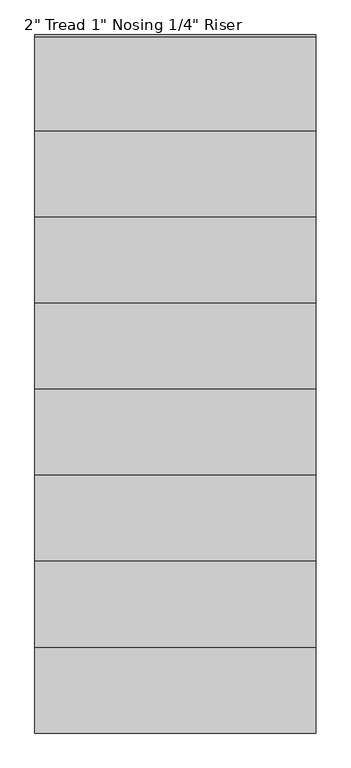
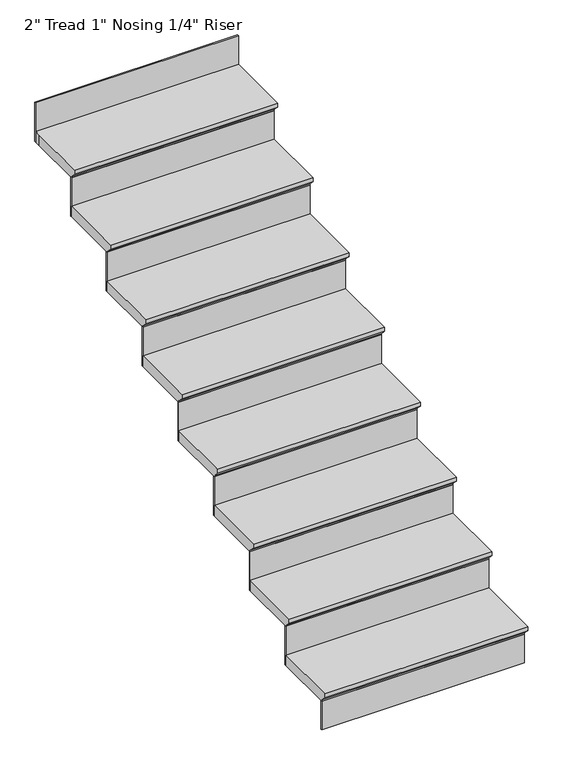
"""IFC4 building model written with IfcOpenShell, lengths in millimetres: stair flight geometry."""

from ifc_helpers import new_model, si_unit, origin, place, context, project, spatial, faceted_brep, source, transform, mapped, element, save


def stair_flight_c2955f1a(model_context):
    return source(origin(), model_context, "Body", "Brep", [
        faceted_brep([(-6758.2994093, 3499.0237487, 167.9863636), (-6758.2994093, 3499.0237487, 187.0363636), (-7672.6994093, 3499.0237487, 187.0363636), (-7672.6994093, 3499.0237487, 167.9863636), (-6758.2994093, 3524.4237487, 142.5863636), (-7672.6994093, 3524.4237487, 142.5863636), (-6758.2994093, 3803.8237487, 187.0363636), (-7672.6994093, 3803.8237487, 187.0363636), (-7672.6994093, 3524.4237487, 136.2363636), (-7672.6994093, 3803.8237487, 136.2363636), (-6758.2994093, 3803.8237487, 136.2363636), (-6758.2994093, 3524.4237487, 136.2363636)], [[[0, 1, 2, 3]], [[4, 0, 3, 5]], [[2, 1, 6, 7]], [[8, 9, 10, 11]], [[2, 7, 9, 8, 5, 3]], [[8, 11, 4, 5]], [[6, 1, 0, 4, 11, 10]], [[7, 6, 10, 9]]]),
        faceted_brep([(-6758.2994093, 3524.4237487, 136.2363636), (-6758.2994093, 3524.4237487, 0.0), (-6758.2994093, 3530.7737487, 0.0), (-6758.2994093, 3530.7737487, 136.2363636), (-7672.6994093, 3524.4237487, 136.2363636), (-7672.6994093, 3530.7737487, 136.2363636), (-7672.6994093, 3530.7737487, 0.0), (-7672.6994093, 3524.4237487, 0.0)], [[[0, 1, 2, 3]], [[4, 5, 6, 7]], [[1, 0, 4, 7]], [[2, 1, 7, 6]], [[3, 2, 6, 5]], [[0, 3, 5, 4]]]),
        faceted_brep([(-6758.2994093, 3803.8237487, 323.2727273), (-6758.2994093, 3803.8237487, 136.2363636), (-6758.2994093, 3810.1737487, 136.2363636), (-6758.2994093, 3810.1737487, 323.2727273), (-7672.6994093, 3803.8237487, 323.2727273), (-7672.6994093, 3810.1737487, 323.2727273), (-7672.6994093, 3810.1737487, 136.2363636), (-7672.6994093, 3803.8237487, 136.2363636)], [[[0, 1, 2, 3]], [[4, 5, 6, 7]], [[1, 0, 4, 7]], [[2, 1, 7, 6]], [[3, 2, 6, 5]], [[0, 3, 5, 4]]]),
        faceted_brep([(-7672.6994093, 3778.4237487, 374.0727273), (-6758.2994093, 3778.4237487, 374.0727273), (-6758.2994093, 4083.2237487, 374.0727273), (-7672.6994093, 4083.2237487, 374.0727273), (-7672.6994093, 3803.8237487, 323.2727273), (-7672.6994093, 4083.2237487, 323.2727273), (-6758.2994093, 4083.2237487, 323.2727273), (-6758.2994093, 3803.8237487, 323.2727273), (-7672.6994093, 3803.8237487, 329.6227273), (-7672.6994093, 3778.4237487, 355.0227273), (-6758.2994093, 3803.8237487, 329.6227273), (-6758.2994093, 3778.4237487, 355.0227273)], [[[0, 1, 2, 3]], [[4, 5, 6, 7]], [[0, 3, 5, 4, 8, 9]], [[4, 7, 10, 8]], [[2, 1, 11, 10, 7, 6]], [[3, 2, 6, 5]], [[11, 1, 0, 9]], [[10, 11, 9, 8]]]),
        faceted_brep([(-6758.2994093, 4083.2237487, 510.3090909), (-6758.2994093, 4083.2237487, 323.2727273), (-6758.2994093, 4089.5737487, 323.2727273), (-6758.2994093, 4089.5737487, 510.3090909), (-7672.6994093, 4083.2237487, 510.3090909), (-7672.6994093, 4089.5737487, 510.3090909), (-7672.6994093, 4089.5737487, 323.2727273), (-7672.6994093, 4083.2237487, 323.2727273)], [[[0, 1, 2, 3]], [[4, 5, 6, 7]], [[1, 0, 4, 7]], [[2, 1, 7, 6]], [[3, 2, 6, 5]], [[0, 3, 5, 4]]]),
        faceted_brep([(-7672.6994093, 4057.8237487, 561.1090909), (-6758.2994093, 4057.8237487, 561.1090909), (-6758.2994093, 4362.6237487, 561.1090909), (-7672.6994093, 4362.6237487, 561.1090909), (-7672.6994093, 4083.2237487, 510.3090909), (-7672.6994093, 4362.6237487, 510.3090909), (-6758.2994093, 4362.6237487, 510.3090909), (-6758.2994093, 4083.2237487, 510.3090909), (-7672.6994093, 4083.2237487, 516.6590909), (-7672.6994093, 4057.8237487, 542.0590909), (-6758.2994093, 4083.2237487, 516.6590909), (-6758.2994093, 4057.8237487, 542.0590909)], [[[0, 1, 2, 3]], [[4, 5, 6, 7]], [[0, 3, 5, 4, 8, 9]], [[4, 7, 10, 8]], [[2, 1, 11, 10, 7, 6]], [[3, 2, 6, 5]], [[11, 1, 0, 9]], [[10, 11, 9, 8]]]),
        faceted_brep([(-6758.2994093, 4362.6237487, 697.3454545), (-6758.2994093, 4362.6237487, 510.3090909), (-6758.2994093, 4368.9737487, 510.3090909), (-6758.2994093, 4368.9737487, 697.3454545), (-7672.6994093, 4362.6237487, 697.3454545), (-7672.6994093, 4368.9737487, 697.3454545), (-7672.6994093, 4368.9737487, 510.3090909), (-7672.6994093, 4362.6237487, 510.3090909)], [[[0, 1, 2, 3]], [[4, 5, 6, 7]], [[1, 0, 4, 7]], [[2, 1, 7, 6]], [[3, 2, 6, 5]], [[0, 3, 5, 4]]]),
        faceted_brep([(-7672.6994093, 4337.2237487, 748.1454545), (-6758.2994093, 4337.2237487, 748.1454545), (-6758.2994093, 4642.0237487, 748.1454545), (-7672.6994093, 4642.0237487, 748.1454545), (-7672.6994093, 4362.6237487, 697.3454545), (-7672.6994093, 4642.0237487, 697.3454545), (-6758.2994093, 4642.0237487, 697.3454545), (-6758.2994093, 4362.6237487, 697.3454545), (-7672.6994093, 4362.6237487, 703.6954545), (-7672.6994093, 4337.2237487, 729.0954545), (-6758.2994093, 4362.6237487, 703.6954545), (-6758.2994093, 4337.2237487, 729.0954545)], [[[0, 1, 2, 3]], [[4, 5, 6, 7]], [[0, 3, 5, 4, 8, 9]], [[4, 7, 10, 8]], [[2, 1, 11, 10, 7, 6]], [[3, 2, 6, 5]], [[11, 1, 0, 9]], [[10, 11, 9, 8]]]),
        faceted_brep([(-6758.2994093, 4642.0237487, 884.3818182), (-6758.2994093, 4642.0237487, 697.3454545), (-6758.2994093, 4648.3737487, 697.3454545), (-6758.2994093, 4648.3737487, 884.3818182), (-7672.6994093, 4642.0237487, 884.3818182), (-7672.6994093, 4648.3737487, 884.3818182), (-7672.6994093, 4648.3737487, 697.3454545), (-7672.6994093, 4642.0237487, 697.3454545)], [[[0, 1, 2, 3]], [[4, 5, 6, 7]], [[1, 0, 4, 7]], [[2, 1, 7, 6]], [[3, 2, 6, 5]], [[0, 3, 5, 4]]]),
        faceted_brep([(-7672.6994093, 4616.6237487, 935.1818182), (-6758.2994093, 4616.6237487, 935.1818182), (-6758.2994093, 4921.4237487, 935.1818182), (-7672.6994093, 4921.4237487, 935.1818182), (-7672.6994093, 4642.0237487, 884.3818182), (-7672.6994093, 4921.4237487, 884.3818182), (-6758.2994093, 4921.4237487, 884.3818182), (-6758.2994093, 4642.0237487, 884.3818182), (-7672.6994093, 4642.0237487, 890.7318182), (-7672.6994093, 4616.6237487, 916.1318182), (-6758.2994093, 4642.0237487, 890.7318182), (-6758.2994093, 4616.6237487, 916.1318182)], [[[0, 1, 2, 3]], [[4, 5, 6, 7]], [[0, 3, 5, 4, 8, 9]], [[4, 7, 10, 8]], [[2, 1, 11, 10, 7, 6]], [[3, 2, 6, 5]], [[11, 1, 0, 9]], [[10, 11, 9, 8]]]),
        faceted_brep([(-6758.2994093, 4921.4237487, 1071.4181818), (-6758.2994093, 4921.4237487, 884.3818182), (-6758.2994093, 4927.7737487, 884.3818182), (-6758.2994093, 4927.7737487, 1071.4181818), (-7672.6994093, 4921.4237487, 1071.4181818), (-7672.6994093, 4927.7737487, 1071.4181818), (-7672.6994093, 4927.7737487, 884.3818182), (-7672.6994093, 4921.4237487, 884.3818182)], [[[0, 1, 2, 3]], [[4, 5, 6, 7]], [[1, 0, 4, 7]], [[2, 1, 7, 6]], [[3, 2, 6, 5]], [[0, 3, 5, 4]]]),
        faceted_brep([(-7672.6994093, 4896.0237487, 1122.2181818), (-6758.2994093, 4896.0237487, 1122.2181818), (-6758.2994093, 5200.8237487, 1122.2181818), (-7672.6994093, 5200.8237487, 1122.2181818), (-7672.6994093, 4921.4237487, 1071.4181818), (-7672.6994093, 5200.8237487, 1071.4181818), (-6758.2994093, 5200.8237487, 1071.4181818), (-6758.2994093, 4921.4237487, 1071.4181818), (-7672.6994093, 4921.4237487, 1077.7681818), (-7672.6994093, 4896.0237487, 1103.1681818), (-6758.2994093, 4921.4237487, 1077.7681818), (-6758.2994093, 4896.0237487, 1103.1681818)], [[[0, 1, 2, 3]], [[4, 5, 6, 7]], [[0, 3, 5, 4, 8, 9]], [[4, 7, 10, 8]], [[2, 1, 11, 10, 7, 6]], [[3, 2, 6, 5]], [[11, 1, 0, 9]], [[10, 11, 9, 8]]]),
        faceted_brep([(-6758.2994093, 5200.8237487, 1258.4545455), (-6758.2994093, 5200.8237487, 1071.4181818), (-6758.2994093, 5207.1737487, 1071.4181818), (-6758.2994093, 5207.1737487, 1258.4545455), (-7672.6994093, 5200.8237487, 1258.4545455), (-7672.6994093, 5207.1737487, 1258.4545455), (-7672.6994093, 5207.1737487, 1071.4181818), (-7672.6994093, 5200.8237487, 1071.4181818)], [[[0, 1, 2, 3]], [[4, 5, 6, 7]], [[1, 0, 4, 7]], [[2, 1, 7, 6]], [[3, 2, 6, 5]], [[0, 3, 5, 4]]]),
        faceted_brep([(-7672.6994093, 5175.4237487, 1309.2545455), (-6758.2994093, 5175.4237487, 1309.2545455), (-6758.2994093, 5480.2237487, 1309.2545455), (-7672.6994093, 5480.2237487, 1309.2545455), (-7672.6994093, 5200.8237487, 1258.4545455), (-7672.6994093, 5480.2237487, 1258.4545455), (-6758.2994093, 5480.2237487, 1258.4545455), (-6758.2994093, 5200.8237487, 1258.4545455), (-7672.6994093, 5200.8237487, 1264.8045455), (-7672.6994093, 5175.4237487, 1290.2045455), (-6758.2994093, 5200.8237487, 1264.8045455), (-6758.2994093, 5175.4237487, 1290.2045455)], [[[0, 1, 2, 3]], [[4, 5, 6, 7]], [[0, 3, 5, 4, 8, 9]], [[4, 7, 10, 8]], [[2, 1, 11, 10, 7, 6]], [[3, 2, 6, 5]], [[11, 1, 0, 9]], [[10, 11, 9, 8]]]),
        faceted_brep([(-6758.2994093, 5759.6237487, 1632.5272727), (-6758.2994093, 5759.6237487, 1445.4909091), (-6758.2994093, 5765.9737487, 1445.4909091), (-6758.2994093, 5765.9737487, 1632.5272727), (-7672.6994093, 5759.6237487, 1632.5272727), (-7672.6994093, 5765.9737487, 1632.5272727), (-7672.6994093, 5765.9737487, 1445.4909091), (-7672.6994093, 5759.6237487, 1445.4909091)], [[[0, 1, 2, 3]], [[4, 5, 6, 7]], [[1, 0, 4, 7]], [[2, 1, 7, 6]], [[3, 2, 6, 5]], [[0, 3, 5, 4]]]),
        faceted_brep([(-6758.2994093, 5480.2237487, 1445.4909091), (-6758.2994093, 5480.2237487, 1258.4545455), (-6758.2994093, 5486.5737487, 1258.4545455), (-6758.2994093, 5486.5737487, 1445.4909091), (-7672.6994093, 5480.2237487, 1445.4909091), (-7672.6994093, 5486.5737487, 1445.4909091), (-7672.6994093, 5486.5737487, 1258.4545455), (-7672.6994093, 5480.2237487, 1258.4545455)], [[[0, 1, 2, 3]], [[4, 5, 6, 7]], [[1, 0, 4, 7]], [[2, 1, 7, 6]], [[3, 2, 6, 5]], [[0, 3, 5, 4]]]),
        faceted_brep([(-7672.6994093, 5759.6237487, 1496.2909091), (-7672.6994093, 5734.2237487, 1496.2909091), (-7672.6994093, 5454.8237487, 1496.2909091), (-6758.2994093, 5454.8237487, 1496.2909091), (-6758.2994093, 5759.6237487, 1496.2909091), (-7672.6994093, 5734.2237487, 1445.4909091), (-7672.6994093, 5759.6237487, 1445.4909091), (-6758.2994093, 5759.6237487, 1445.4909091), (-6758.2994093, 5480.2237487, 1445.4909091), (-7672.6994093, 5480.2237487, 1445.4909091), (-7672.6994093, 5480.2237487, 1451.8409091), (-7672.6994093, 5454.8237487, 1477.2409091), (-6758.2994093, 5480.2237487, 1451.8409091), (-6758.2994093, 5454.8237487, 1477.2409091)], [[[0, 1, 2, 3, 4]], [[5, 6, 7, 8, 9]], [[1, 0, 6, 5]], [[2, 1, 5, 9, 10, 11]], [[9, 8, 12, 10]], [[4, 3, 13, 12, 8, 7]], [[0, 4, 7, 6]], [[13, 3, 2, 11]], [[12, 13, 11, 10]]]),
    ])


if __name__ == "__main__":
    model = new_model("IFC4")
    model_context = context("Model", 3, world=origin())
    ifc_project = project(units=[si_unit("LENGTHUNIT", "METRE", prefix="MILLI")], contexts=[model_context])
    site = spatial("IfcSite", under=ifc_project)
    building = spatial("IfcBuilding", under=site)
    placement = place(None, origin())
    stair_flight_shape = stair_flight_c2955f1a(model_context)
    element("IfcStairFlight", 1, ObjectType="2\" Tread 1\" Nosing 1/4\" Riser", at=placement, inside=building, context=model_context, shape_type="MappedRepresentation", body=[
        mapped(stair_flight_shape, transform((0.0, 0.0, 0.0), x_axis=(1.0, 0.0, 0.0), y_axis=(0.0, 1.0, 0.0), z_axis=(0.0, 0.0, 1.0))),
    ])
    save(model, "model.ifc")
